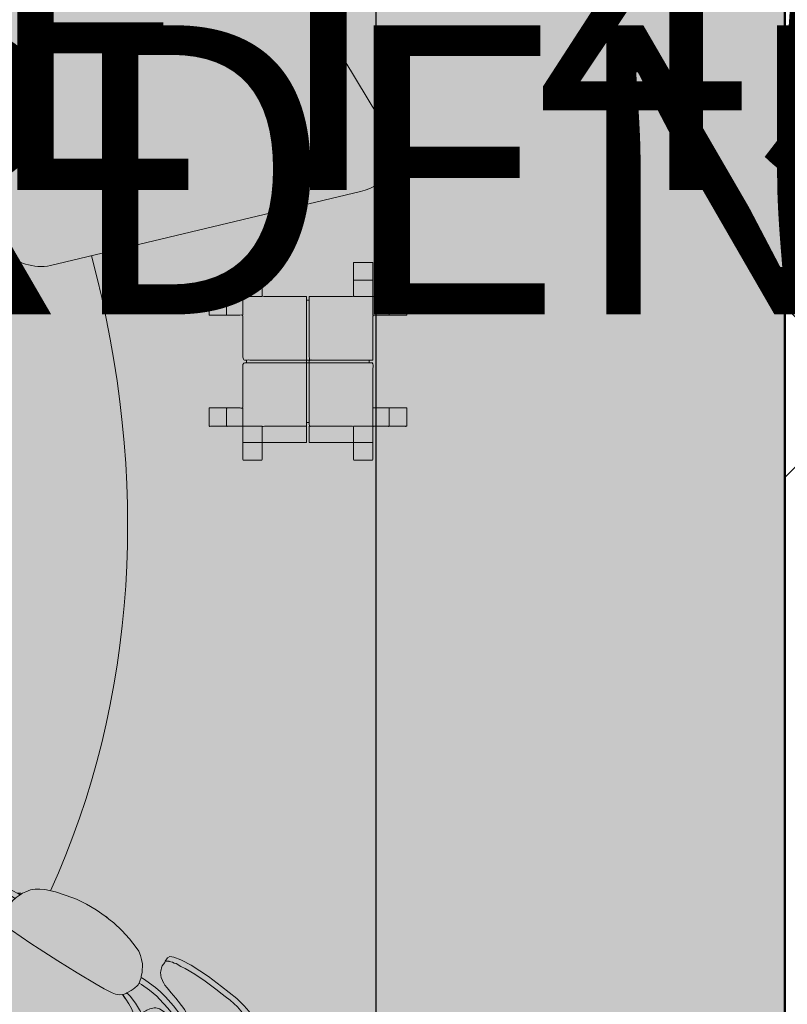
# Model space of a CAD drawing. Units: inches. Extents: x -466983 to 1020, y 324 to 318697.
# Tile 17 of 97: x 797.94 to 813.86, y 452.46 to 472.89. Entities that reach past the tile are written whole.
import ezdxf

# ---------------------------------------------------------------- set-up
doc = ezdxf.new("R2010")
doc.units = ezdxf.units.IN
doc.header["$MEASUREMENT"] = 0
for name, color, linetype, lineweight in [('A-ANNO-DIMS', 2, 'Continuous', 18), ('A-FLOR-PATT', 252, 'Continuous', 13), ('A-FURN', 8, 'Continuous', 18), ('A-WALL', 7, 'Continuous', 50)]:
    doc.layers.add(name, color=color, linetype=linetype, lineweight=lineweight)
doc.layers.add('K-Hatch', color=7, linetype='Continuous')
doc.styles.get("Standard").update_dxf_attribs({"font": 'arial.ttf'})
doc.dimstyles.get("Standard").update_dxf_attribs({"dimtxt": 6, "dimasz": 4, "dimexe": 3, "dimexo": 3, "dimgap": 0.09, "dimtad": 0, "dimtih": 1, "dimtoh": 1, "dimdec": 1, "dimzin": 0, "dimdsep": 46, "dimlunit": 3, "dimtxsty": 'Standard', "dimcen": 0.09, "dimadec": 0, "dimazin": 0, "dimtfac": 1, "dimtdec": 1, "dimtofl": 0, "dimtmove": 0, "dimatfit": 3, "dimfxl": 1, "dimtolj": 1, "dimtzin": 0, "dimarcsym": 0})

# ---------------------------------------------------------------- blocks, each defined once
blk = doc.blocks.new('CBV_09')
for points, knots in [([(-122.8, 153.5), (-122.8, 170.2), (-122.8, 186.8), (-104.5, 186.8), (-86.3, 186.8)], [99, 99, 99, 100, 100, 101, 101, 101]), ([(-122.8, 153.5), (-122.8, 170.2), (-122.8, 186.8), (-104.5, 186.8), (-86.3, 186.8)], [99, 99, 99, 100, 100, 101, 101, 101]), ([(86.3, 153.5), (86.3, 170.2), (86.3, 186.8), (104.5, 186.8), (122.8, 186.8)], [45, 45, 45, 46, 46, 47, 47, 47]), ([(86.3, 153.5), (86.3, 170.2), (86.3, 186.8), (104.5, 186.8), (122.8, 186.8)], [45, 45, 45, 46, 46, 47, 47, 47]), ([(-29.2, 122.7), (-20.7, 122.7), (-12.2, 122.7), (-7.4, 122.7), (-2.6, 122.7), (-2.6, 105.2), (-2.6, 87.7), (-2.6, 45.2), (-2.6, 2.6), (-7.4, 2.6), (-12.2, 2.6), (-20.7, 2.6), (-29.2, 2.6), (-57.8, 2.6), (-86.3, 2.6), (-104.5, 2.6), (-122.8, 2.6), (-122.8, 45.2), (-122.8, 87.7), (-138.1, 87.7), (-153.5, 87.7), (-153.5, 105.2), (-153.5, 122.7), (-138.1, 122.7), (-122.8, 122.7), (-122.8, 138.1), (-122.8, 153.5), (-104.5, 153.5), (-86.3, 153.5), (-86.3, 138.1), (-86.3, 122.7), (-57.8, 122.7), (-29.2, 122.7)], [73, 73, 73, 74, 74, 75, 75, 76, 76, 77, 77, 78, 78, 79, 79, 80, 80, 81, 81, 82, 82, 83, 83, 84, 84, 85, 85, 86, 86, 87, 87, 88, 88, 89, 89, 89]), ([(-29.2, 122.7), (-20.7, 122.7), (-12.2, 122.7), (-7.4, 122.7), (-2.6, 122.7), (-2.6, 105.2), (-2.6, 87.7), (-2.6, 45.2), (-2.6, 2.6), (-7.4, 2.6), (-12.2, 2.6), (-20.7, 2.6), (-29.2, 2.6), (-57.8, 2.6), (-86.3, 2.6), (-104.5, 2.6), (-122.8, 2.6), (-122.8, 45.2), (-122.8, 87.7), (-138.1, 87.7), (-153.5, 87.7), (-153.5, 105.2), (-153.5, 122.7), (-138.1, 122.7), (-122.8, 122.7), (-122.8, 138.1), (-122.8, 153.5), (-104.5, 153.5), (-86.3, 153.5), (-86.3, 138.1), (-86.3, 122.7), (-57.8, 122.7), (-29.2, 122.7)], [73, 73, 73, 74, 74, 75, 75, 76, 76, 77, 77, 78, 78, 79, 79, 80, 80, 81, 81, 82, 82, 83, 83, 84, 84, 85, 85, 86, 86, 87, 87, 88, 88, 89, 89, 89]), ([(29.1, 2.6), (20.6, 2.6), (12.1, 2.6), (7.3, 2.6), (2.6, 2.6), (2.6, 45.2), (2.6, 87.7), (2.6, 105.2), (2.6, 122.7), (7.3, 122.7), (12.1, 122.7), (20.6, 122.7), (29.1, 122.7), (57.7, 122.7), (86.3, 122.7), (86.3, 138.1), (86.3, 153.5), (104.5, 153.5), (122.8, 153.5), (122.8, 138.1), (122.8, 122.7)], [26, 26, 26, 27, 27, 28, 28, 29, 29, 30, 30, 31, 31, 32, 32, 33, 33, 34, 34, 35, 35, 36, 36, 36]), ([(-153.5, 87.7), (-170.2, 87.7), (-186.8, 87.7), (-186.8, 105.2), (-186.8, 122.7)], [110, 110, 110, 111, 111, 112, 112, 112]), ([(-153.5, 87.7), (-170.2, 87.7), (-186.8, 87.7), (-186.8, 105.2), (-186.8, 122.7)], [110, 110, 110, 111, 111, 112, 112, 112]), ([(-122.8, 87.7), (-122.8, 105.2), (-122.8, 122.7), (-104.5, 122.7), (-86.3, 122.7)], [0, 0, 0, 1, 1, 2, 2, 2]), ([(122.8, 122.7), (138.1, 122.7), (153.5, 122.7), (153.5, 105.2), (153.5, 87.7), (138.1, 87.7), (122.8, 87.7), (122.8, 45.2), (122.8, 2.6), (104.5, 2.6), (86.3, 2.6), (57.7, 2.6), (29.1, 2.6)], [324, 324, 324, 325, 325, 326, 326, 327, 327, 328, 328, 329, 329, 330, 330, 330]), ([(122.8, 122.7), (138.1, 122.7), (153.5, 122.7), (153.5, 105.2), (153.5, 87.7), (138.1, 87.7), (122.8, 87.7), (122.8, 45.2), (122.8, 2.6), (104.5, 2.6), (86.3, 2.6), (57.7, 2.6), (29.1, 2.6)], [324, 324, 324, 325, 325, 326, 326, 327, 327, 328, 328, 329, 329, 330, 330, 330]), ([(122.8, 87.7), (122.8, 105.2), (122.8, 122.7), (104.5, 122.7), (86.3, 122.7)], [1, 1, 1, 2, 2, 3, 3, 3]), ([(153.5, 122.7), (170.2, 122.7), (186.8, 122.7), (186.8, 105.2), (186.8, 87.7), (170.2, 87.7), (153.5, 87.7)], [314, 314, 314, 315, 315, 316, 316, 317, 317, 317]), ([(153.5, 122.7), (170.2, 122.7), (186.8, 122.7), (186.8, 105.2), (186.8, 87.7), (170.2, 87.7), (153.5, 87.7)], [314, 314, 314, 315, 315, 316, 316, 317, 317, 317]), ([(-2.6, 2.6), (-2.6, 0), (-2.6, -2.6), (0, -2.6), (2.6, -2.6)], [0.000014, 0.000014, 0.000014, 1, 1, 2, 2, 2]), ([(2.6, -2.6), (2.6, 0), (2.6, 2.6), (0, 2.6), (-2.6, 2.6)], [2, 2, 2, 3, 3, 3.999968, 3.999968, 3.999968]), ([(-122.8, -122.7), (-138.1, -122.7), (-153.5, -122.7), (-153.5, -105.2), (-153.5, -87.7), (-138.1, -87.7), (-122.8, -87.7), (-122.8, -45.2), (-122.8, -2.6), (-104.5, -2.6), (-86.3, -2.6), (-57.8, -2.6), (-29.2, -2.6), (-20.7, -2.6), (-12.2, -2.6), (-7.4, -2.6), (-2.6, -2.6)], [0, 0, 0, 1, 1, 2, 2, 3, 3, 4, 4, 5, 5, 6, 6, 7, 7, 8, 8, 8]), ([(-122.8, -122.7), (-138.1, -122.7), (-153.5, -122.7), (-153.5, -105.2), (-153.5, -87.7), (-138.1, -87.7), (-122.8, -87.7), (-122.8, -45.2), (-122.8, -2.6), (-104.5, -2.6), (-86.3, -2.6), (-57.8, -2.6), (-29.2, -2.6), (-20.7, -2.6), (-12.2, -2.6), (-7.4, -2.6), (-2.6, -2.6)], [0, 0, 0, 1, 1, 2, 2, 3, 3, 4, 4, 5, 5, 6, 6, 7, 7, 8, 8, 8]), ([(-2.6, -2.6), (-2.6, -45.2), (-2.6, -87.7), (-2.6, -105.2), (-2.6, -122.7), (-7.4, -122.7), (-12.2, -122.7), (-20.7, -122.7), (-29.2, -122.7), (-57.8, -122.7), (-86.3, -122.7), (-86.3, -138.1), (-86.3, -153.5), (-104.5, -153.5), (-122.8, -153.5), (-122.8, -138.1), (-122.8, -122.7)], [344, 344, 344, 345, 345, 346, 346, 347, 347, 348, 348, 349, 349, 350, 350, 351, 351, 352, 352, 352]), ([(153.5, -87.7), (153.5, -105.2), (153.5, -122.7), (138.1, -122.7), (122.8, -122.7), (122.8, -138.1), (122.8, -153.5), (104.5, -153.5), (86.3, -153.5), (86.3, -138.1), (86.3, -122.7), (57.7, -122.7), (29.1, -122.7), (20.6, -122.7), (12.1, -122.7), (7.3, -122.7), (2.6, -122.7), (2.6, -105.2), (2.6, -87.7), (2.6, -45.2), (2.6, -2.6), (7.3, -2.6), (12.1, -2.6), (20.6, -2.6), (29.1, -2.6), (57.7, -2.6), (86.3, -2.6), (104.5, -2.6), (122.8, -2.6), (122.8, -45.2), (122.8, -87.7)], [279.000001, 279.000001, 279.000001, 280, 280, 281, 281, 282, 282, 283, 283, 284, 284, 285, 285, 286, 286, 287, 287, 288, 288, 289, 289, 290, 290, 291, 291, 292, 292, 293, 293, 294, 294, 294]), ([(-153.5, -122.7), (-170.2, -122.7), (-186.8, -122.7), (-186.8, -105.2), (-186.8, -87.7)], [150, 150, 150, 151, 151, 152, 152, 152]), ([(-153.5, -122.7), (-170.2, -122.7), (-186.8, -122.7), (-186.8, -105.2), (-186.8, -87.7)], [150, 150, 150, 151, 151, 152, 152, 152]), ([(-122.8, -87.7), (-122.8, -105.2), (-122.8, -122.7), (-104.5, -122.7), (-86.3, -122.7)], [1, 1, 1, 2, 2, 3, 3, 3]), ([(122.8, -87.7), (122.8, -105.2), (122.8, -122.7), (104.5, -122.7), (86.3, -122.7)], [1, 1, 1, 2, 2, 3, 3, 3]), ([(153.5, -87.7), (170.2, -87.7), (186.8, -87.7), (186.8, -105.2), (186.8, -122.7), (170.2, -122.7), (153.5, -122.7)], [238, 238, 238, 239, 239, 240, 240, 241, 241, 241]), ([(153.5, -87.7), (170.2, -87.7), (186.8, -87.7), (186.8, -105.2), (186.8, -122.7), (170.2, -122.7), (153.5, -122.7)], [238, 238, 238, 239, 239, 240, 240, 241, 241, 241]), ([(-86.3, -153.5), (-86.3, -170.2), (-86.3, -186.8), (-104.5, -186.8), (-122.8, -186.8), (-122.8, -170.2), (-122.8, -153.5)], [161, 161, 161, 162, 162, 163, 163, 164, 164, 164]), ([(-86.3, -153.5), (-86.3, -170.2), (-86.3, -186.8), (-104.5, -186.8), (-122.8, -186.8), (-122.8, -170.2), (-122.8, -153.5)], [161, 161, 161, 162, 162, 163, 163, 164, 164, 164]), ([(-2.6, -153.5), (-7.4, -153.5), (-12.2, -153.5), (-20.7, -153.5), (-29.2, -153.5), (-57.8, -153.5), (-86.3, -153.5)], [258, 258, 258, 259, 259, 260, 260, 261, 261, 261]), ([(-2.6, -153.5), (-7.4, -153.5), (-12.2, -153.5), (-20.7, -153.5), (-29.2, -153.5), (-57.8, -153.5), (-86.3, -153.5)], [258, 258, 258, 259, 259, 260, 260, 261, 261, 261]), ([(86.3, -153.5), (57.7, -153.5), (29.1, -153.5), (20.6, -153.5), (12.1, -153.5), (7.3, -153.5), (2.6, -153.5)], [254, 254, 254, 255, 255, 256, 256, 257, 257, 257]), ([(86.3, -153.5), (57.7, -153.5), (29.1, -153.5), (20.6, -153.5), (12.1, -153.5), (7.3, -153.5), (2.6, -153.5)], [254, 254, 254, 255, 255, 256, 256, 257, 257, 257]), ([(122.8, -153.5), (122.8, -170.2), (122.8, -186.8), (104.5, -186.8), (86.3, -186.8), (86.3, -170.2), (86.3, -153.5)], [227, 227, 227, 228, 228, 229, 229, 230, 230, 230]), ([(122.8, -153.5), (122.8, -170.2), (122.8, -186.8), (104.5, -186.8), (86.3, -186.8), (86.3, -170.2), (86.3, -153.5)], [227, 227, 227, 228, 228, 229, 229, 230, 230, 230])]:
    blk.add_open_spline(points, degree=2, knots=knots)
for points in [[(-86.3, 186.8), (-86.3, 170.2), (-86.3, 153.5)], [(-86.3, 186.8), (-86.3, 170.2), (-86.3, 153.5)], [(122.8, 186.8), (122.8, 170.2), (122.8, 153.5)], [(122.8, 186.8), (122.8, 170.2), (122.8, 153.5)], [(-186.8, 122.7), (-170.2, 122.7), (-153.5, 122.7)], [(-186.8, 122.7), (-170.2, 122.7), (-153.5, 122.7)], [(-2.6, 115.7), (0, 115.7), (2.6, 115.7)], [(-2.6, 115.7), (0, 115.7), (2.6, 115.7)], [(2.6, 122.7), (2.6, 122.7), (2.6, 122.7)], [(2.6, 122.7), (2.6, 122.7), (2.6, 122.7)], [(-115.7, -2.6), (-115.7, 0), (-115.7, 2.6)], [(-115.7, -2.6), (-115.7, 0), (-115.7, 2.6)], [(-2.6, 2.6), (-2.6, 2.6), (-2.6, 2.6)], [(-2.6, 2.6), (-2.6, 2.6), (-2.6, 2.6)], [(115.7, 2.6), (115.7, 0), (115.7, -2.6)], [(115.7, 2.6), (115.7, 0), (115.7, -2.6)], [(115.7, 2.6), (119.2, 2.6), (122.8, 2.6)], [(115.7, 2.6), (119.2, 2.6), (122.8, 2.6)], [(-86.3, -2.6), (-86.3, -2.6), (-86.3, -2.6)], [(-86.3, -2.6), (-86.3, -2.6), (-86.3, -2.6)], [(-29.2, -2.6), (-29.2, -2.6), (-29.2, -2.6)], [(-29.2, -2.6), (-29.2, -2.6), (-29.2, -2.6)], [(-12.2, -2.6), (-12.2, -2.6), (-12.2, -2.6)], [(-12.2, -2.6), (-12.2, -2.6), (-12.2, -2.6)], [(2.6, -2.6), (2.6, -2.6), (2.6, -2.6)], [(12.1, -2.6), (12.1, -2.6), (12.1, -2.6)], [(12.1, -2.6), (12.1, -2.6), (12.1, -2.6)], [(29.1, -2.6), (29.1, -2.6), (29.1, -2.6)], [(86.3, -2.6), (86.3, -2.6), (86.3, -2.6)], [(86.3, -2.6), (86.3, -2.6), (86.3, -2.6)], [(115.7, -2.6), (115.7, -2.6), (115.7, -2.6)], [(115.7, -2.6), (115.7, -2.6), (115.7, -2.6)], [(115.7, -2.6), (119.2, -2.6), (122.8, -2.6)], [(115.7, -2.6), (119.2, -2.6), (122.8, -2.6)], [(-186.8, -87.7), (-170.2, -87.7), (-153.5, -87.7)], [(-186.8, -87.7), (-170.2, -87.7), (-153.5, -87.7)], [(122.8, -87.7), (138.1, -87.7), (153.5, -87.7)], [(122.8, -87.7), (138.1, -87.7), (153.5, -87.7)], [(2.6, -115.7), (0, -115.7), (-2.6, -115.7)], [(-2.6, -153.5), (-2.6, -138.1), (-2.6, -122.7)], [(2.6, -153.5), (2.6, -138.1), (2.6, -122.7)]]:
    blk.add_open_spline(points, degree=2)
blk = doc.blocks.new('CBV_05')
at = {"layer": 'K-Hatch'}
h = blk.add_hatch(color=256, dxfattribs=at)
h.dxf.hatch_style = 1
h.paths.add_polyline_path([(614, 437), (1251.4, 62.5), (1198.3, -263.2), (564.8, -9.8), (344.4, -5.5), (343.7, -629.7, 0.159768), (369.9, -672.6), (1020.5, -1025.6, 0.317347), (1135.5, -1017.7), (1739.5, -492.7, 0.378101), (1761.2, -362.2), (1507.4, -70.4, -0.119239), (1492.6, -25.8), (1499.5, 665.1, 0.256804), (1446.2, 745.4), (822.7, 1028.7, 0.297137), (714, 1018.3), (625, 963.6), (549.5, 1037.1), (186.8, 587.5), (-1106.2, 397.7), (-1098.6, 311.5), (-1098.4, 310.2)])
h.paths.add_polyline_path([(344.4, -5.5), (-1216.9, 24.6), (-1212.3, 260), (-1718.1, 162.7, 0.51466), (-1765.1, 50), (-1478.1, -479.5, 0.244482), (-1398.8, -526.6), (323.6, -658.2, 0.453292), (343.1, -629.8, 0.006511), (343.7, -631.8)])
blk.add_lwpolyline([(1761.2, -362.2, -0.378101), (1739.5, -492.7), (1135.5, -1017.7, -0.317347), (1020.5, -1025.6), (369.9, -672.6, -0.159481), (343.2, -630.1, -0.449095), (323.6, -658.2), (-1398.8, -526.6, -0.244482), (-1478.1, -479.5), (-1765.1, 50, -0.51466), (-1718.1, 162.7), (-1212.3, 260), (-1211.5, 301.9), (-1098.4, 310.2), (-1106.2, 397.7), (186.8, 587.5), (549.5, 1037.1), (625, 963.6), (714, 1018.3, -0.297137), (822.7, 1028.7), (1446.2, 745.4, -0.256804), (1499.5, 665.1), (1492.6, -25.8, 0.119239), (1507.4, -70.4)], format="xyb", close=True)
blk.add_lwpolyline([(-1212.3, 260), (-1718.1, 162.7, 0.51466), (-1765.1, 50), (-1478.1, -479.5, 0.244482), (-1398.8, -526.6), (323.6, -658.2)], format="xyb")
blk = doc.blocks.new('CBV_11')
at = {"layer": 'K-Hatch'}
h = blk.add_hatch(color=256, dxfattribs=at)
h.dxf.hatch_style = 1
h.paths.add_polyline_path([(-178.4, 698.3), (-200.4, 717.9), (-207.1, 720), (-213, 721.7), (-231.8, 722.5), (-254.2, 721.5), (-275, 717.7), (-289.3, 712.5), (-316, 699.4), (-324.9, 694.8), (-295.8, 706.5), (-286.8, 709.3), (-277.1, 712.2), (-265.3, 715), (-258.1, 715.9), (-241.3, 718.1), (-228.8, 718), (-215.5, 715.7), (-208.8, 713.2), (-205.5, 711.6), (-203.9, 710.6), (-202.4, 709.7), (-195.4, 705.2), (-194.8, 704.5), (-190.4, 699.8), (-87.3, 570), (16.1, 440.3), (19.6, 435), (22.9, 426.4), (24.1, 422.9), (25.8, 412.3), (25.1, 398.9), (24.2, 394.5), (25.6, 399.8), (28.8, 418.8), (27.5, 432), (13.6, 457)])
h.paths.add_polyline_path([(-536, 213.1), (-639.3, 342.7), (-642.9, 348.1), (-646.2, 356.7), (-647.4, 360.2), (-649.1, 370.8), (-648.4, 384.2), (-645.7, 396.4), (-637.3, 419.1), (-631.8, 430), (-626.9, 438.8), (-622.1, 446.9), (-606.5, 469.3), (-631, 439.9), (-638.6, 427.4), (-646.5, 408.6), (-652.3, 388), (-655.6, 368.8), (-654.4, 355.7), (-649, 343.1), (-640.5, 330.7), (-448.6, 89.4), (-437.6, 77.7), (-424.8, 69.2), (-413.8, 65.9), (-392.4, 64.7), (-388.1, 65), (-394.5, 65), (-407.8, 67.4), (-417, 71.1), (-420.9, 73.4), (-427.9, 77.9), (-428.5, 78.6), (-432.9, 83.2)])
for p, q in [((259, 150.4), (259, 150.4)), ((345.2, 98.6), (344, 99.3)), ((349.3, 96), (349.2, 96.1)), ((478.6, -6.2), (478.7, -6.3)), ((644.9, -391.7), (644.8, -391.9)), ((-99, -470.6), (-98.6, -470.7)), ((4, -570.8), (3.9, -570.4)), ((96.9, -581.8), (98.6, -582.5)), ((157.6, -594.8), (157.4, -595)), ((239.9, -716.7), (240.2, -716.7))]:
    blk.add_line(p, q)
for points in [[(9, 353), (10.3, 354.9), (16.2, 365.1), (21.5, 376.3), (26.2, 388.3), (30.1, 400.3), (33.2, 412.3), (35.5, 424.1), (35.7, 431), (33.5, 442.1), (26.2, 456.4), (21.3, 463.1), (-173.2, 707.5), (-185, 718.7), (-200.1, 726), (-205.3, 726.9), (-216.4, 727.2), (-226.1, 726.9), (-241.2, 725.8), (-253.7, 723.9), (-264.9, 721.5), (-277.2, 717.9), (-288.3, 713.3), (-311.8, 701.8), (-324.9, 694.8), (-316, 699.4), (-289.3, 712.5), (-275, 717.7), (-254.2, 721.5), (-231.8, 722.5), (-213, 721.7), (-207.1, 720), (-200.4, 717.9), (-178.4, 698.3), (13.6, 457), (27.5, 432), (28.8, 418.8), (25.6, 399.8), (24.2, 394.5)], [(-16.4, 313.8), (-16.1, 314.2), (2.3, 340.9), (8.8, 352.7), (9, 353), (14.8, 365.2), (18.6, 375.8), (20.5, 381.1), (22.4, 386.6), (24.2, 394.5), (25.1, 398.9), (25.8, 412.3), (24.1, 422.9), (22.9, 426.4), (19.6, 435), (16.1, 440.3), (-87.3, 570), (-190.4, 699.8), (-194.8, 704.5), (-195.4, 705.2), (-202.4, 709.7), (-203.9, 710.6), (-208.8, 713.2), (-215.5, 715.7), (-228.8, 718), (-241.3, 718.1), (-258.1, 715.9), (-265.3, 715), (-277.1, 712.2), (-286.8, 709.3), (-295.8, 706.5), (-324.9, 694.8), (-347.4, 685.7), (-397.3, 660.4), (-444.8, 630.8), (-480.8, 604.2), (-497.4, 590.5), (-534.5, 556.2), (-554.4, 535.5), (-590.2, 492.6), (-603.5, 473.5), (-606.5, 469.3), (-622.1, 446.9), (-626.9, 438.8), (-631.8, 430), (-637.3, 419.1), (-645.7, 396.4), (-648.4, 384.2), (-649.1, 370.8), (-647.4, 360.2), (-646.2, 356.7), (-642.9, 348.1), (-639.3, 342.7), (-536, 213.1), (-432.9, 83.2), (-428.5, 78.6), (-427.9, 77.9), (-420.9, 73.4), (-417, 71.1), (-407.8, 67.4), (-394.5, 65), (-388.1, 65), (-382, 64.9), (-376.6, 65.6), (-368.3, 66.6), (-367.7, 66.7), (-359.3, 67.5), (-346.5, 70.4), (-345.9, 70.6), (-336.1, 73.3), (-327.3, 76.2), (-282.4, 94.4), (-275.6, 97.1), (-225.7, 122.4), (-178.3, 151.9), (-142.2, 178.6), (-125.6, 192.2), (-88.5, 226.6), (-68.7, 247.3), (-32.9, 290.2), (-16.4, 313.8), (-16.2, 314.2)], [(-203.9, 710.6), (-205.5, 711.6), (-208.8, 713.2)], [(-346.5, 70.4), (-349.3, 69.2), (-356.8, 67), (-372.9, 63.3), (-385.5, 61.5), (-398.1, 60.5), (-410.3, 60.2), (-421.5, 60.6), (-428.5, 61.9), (-441.8, 68.9), (-453.7, 80.2), (-456.3, 83.2), (-648.2, 324.6), (-653.1, 331.3), (-657.2, 338.3), (-662.3, 353.4), (-662.3, 363.4), (-659.9, 375.1), (-656.8, 387), (-652.8, 399), (-648.1, 410.9), (-642.7, 422.1), (-636.8, 432.3), (-630.4, 441.2), (-607, 469.6), (-603.5, 473.5)], [(-606.5, 469.3), (-631, 439.9), (-638.6, 427.4), (-646.5, 408.6), (-652.3, 388), (-655.6, 368.8), (-654.4, 355.7), (-649, 343.1), (-640.5, 330.7), (-448.6, 89.4), (-437.6, 77.7), (-424.8, 69.2), (-413.8, 65.9), (-392.4, 64.7), (-388.1, 65)], [(-50.1, 67.5), (-23.5, 87.9), (-9.9, 97.6), (3.8, 107.1), (17.8, 116.4), (31.9, 125.3), (60.6, 142.4), (89.9, 158.3), (119.5, 173.3), (135, 179.9), (142.8, 182.8), (151, 184.8), (159.6, 185.9), (175.9, 186.9), (181, 186.7)], [(46.8, 133.3), (53.6, 137.3), (58.1, 140), (60.8, 141.6), (71.5, 147.3), (71.5, 147.3), (75.4, 149.5), (86.9, 155.7), (90, 157.4), (100.5, 162.5), (100.5, 162.6), (112.3, 168.5), (118.5, 171.5), (121.5, 172.9), (121.5, 172.9), (121.6, 172.9), (124.8, 174.4), (126.7, 175.2), (131.7, 177.5), (133.5, 178.2), (133.6, 178.2), (139.5, 180.3), (143.1, 181.6), (144.9, 182), (148.5, 182.9), (151.1, 183.5), (151.4, 183.6), (155.5, 184.6), (157.4, 184.8), (163.9, 185.7), (168.2, 186.2), (170.2, 186.3), (175.4, 186.4), (175.6, 186.4), (175.8, 186.4), (179.6, 186.5), (181.7, 186.3), (187.4, 185.9), (192.1, 185.5), (192.4, 185.5), (192.9, 185.4), (196.6, 184.9), (199.1, 184.5), (203, 183.5), (203.6, 183.4), (204.9, 183.1), (206.1, 182.8), (206.2, 182.8), (206.9, 182.5), (210.6, 181.4), (212.8, 180.8), (213.1, 180.7), (213.6, 180.5), (215.8, 179.8), (217.2, 179.4), (219, 178.7), (225, 176.1), (225.2, 176), (225.4, 175.9), (228.9, 174.4), (230.6, 173.5), (239.3, 168.6), (259, 150.4), (261.9, 146.4), (265.2, 141.7), (271.3, 132.8), (271.8, 133.4)], [(268, 169.8), (264.7, 172.2), (256.3, 176.5), (245.7, 180.3), (233.5, 183.5), (219.5, 185.8), (204.9, 187.1), (190.5, 187.3), (181, 186.7), (184.6, 186.6), (192.1, 185.5)], [(215.8, 179.8), (224.2, 178.5), (244.5, 172), (258.1, 164.6), (259.6, 163.4)], [(325.2, 88.8), (320.7, 95.5), (312.8, 106.8), (299.7, 124.6), (287.2, 140.3), (277.4, 151.6), (268.4, 160.4), (262.4, 164.5), (259.6, 163.6), (268, 169.8), (268.8, 170.4), (273.2, 169.7), (281.2, 162.9), (287.4, 156.5), (292.6, 150.4), (299.8, 141.9), (315.6, 121.4), (329.6, 101.6), (335.5, 92.9)], [(259.6, 163.6), (259.6, 163.4), (260.3, 157.9), (264.5, 147.6), (271, 134.8), (273.6, 130.4), (280, 119.4), (306, 80.1)], [(346.5, 95.7), (344, 99.3), (342.7, 101.1), (342.4, 101.6), (329.1, 118.9), (319.4, 130.1), (312.4, 136.8), (292.6, 150.4)], [(58.1, 140), (55.3, 138.4), (46.8, 133.3), (43.3, 131.2), (32.8, 125), (30.4, 123.5), (28, 122), (23.4, 119.1), (14, 112.9), (5.4, 107.3), (1.3, 104.5), (-2.9, 101.6), (-9.4, 97), (-9.5, 96.9), (-21, 88.8), (-24.8, 86), (-28.5, 83.3), (-36.4, 77.2), (-38.8, 75.4), (-45.1, 70.6), (-49.7, 67), (-54.2, 63.4), (-56, 61.9), (-62.5, 56.6), (-75.5, 45.6), (-77.3, 44), (-77.4, 44)], [(457.4, -155.4), (455.9, -155.5), (454.8, -155.5), (454.6, -155.5), (454.5, -155.5), (450.3, -155.2), (448.8, -154.8), (444.9, -153.5), (441.6, -151.7), (437.3, -148.8), (429.3, -140.4), (425.9, -136.3), (421.6, -130.7), (411.3, -116.8), (398.5, -99.2), (386.7, -82.7), (374.5, -65.3), (362.5, -47.8), (339.1, -12.8), (318.2, 19.8), (307.7, 36.3), (302.4, 46.9), (301.4, 48.8), (298.5, 55.5), (297.9, 58.1), (297.8, 65.2), (298.5, 67.6), (301, 75.1), (306, 80.1), (307.5, 81.6), (308.1, 82), (307.8, 84), (308.9, 85.7), (310.4, 86.8), (312.8, 87.1), (320.3, 87.9), (323, 87.9), (324.8, 88.6), (325.2, 88.8), (330.7, 91.3), (335.5, 92.9), (337.7, 93.7), (344.7, 95.5), (346.5, 95.7), (349.3, 96), (349.8, 96), (359.2, 96.9), (368.2, 95.8), (377.2, 93.8), (385.7, 90.7), (393.6, 86.2), (410.4, 73.5), (416, 68.7), (426.3, 59.8), (441.3, 45.2), (454.8, 29), (467.2, 12.1), (478.3, -5.7), (478.6, -6.2), (478.6, -6.3), (479, -7), (481, -10.8), (488.2, -24.1), (496, -43.4), (503.1, -63.4), (508.5, -83.5), (509.8, -91.8), (509.7, -100.3), (508.6, -108.6), (506.6, -116.7), (503.3, -124.2), (500, -131.2), (494.1, -139.1), (490.8, -143.5), (486.4, -147), (485.6, -147.6), (485.6, -147.6)], [(349.8, 96), (347.9, 98), (342.9, 101.1), (342.7, 101.1)], [(-217.7, -216.8), (-218.7, -214.8), (-221.6, -206), (-223.5, -195.1), (-224.4, -170.3), (-223.2, -156.5), (-220.9, -142.4), (-219, -134.5), (-218.9, -134.4), (-218.9, -134.2), (-217.3, -125.9), (-215.2, -117.7), (-212.7, -109.9), (-212.1, -108.4), (-207.7, -98.2), (-203.6, -90.8), (-196.4, -80.6), (-191.3, -74), (-180.9, -61.1), (-170.2, -48.3), (-159.1, -35.9), (-159.1, -35.8), (-148, -23.5), (-124.9, 0.7), (-113, 12.4), (-100.8, 23.9), (-88.5, 35.1), (-75.9, 46.2), (-63.1, 57), (-50.1, 67.5)], [(-214.7, -118), (-214.6, -117.8), (-212.4, -111.4), (-210.9, -107.7), (-210.4, -106.5), (-210.1, -105.7), (-209.4, -104.2), (-209, -103.5), (-206, -97.3), (-205.1, -95.8), (-204.7, -95), (-203.9, -93.8), (-203.5, -93.2), (-202.6, -91.5), (-202, -90.5), (-200.3, -88.1), (-199.3, -86.6), (-198.2, -84.9), (-198, -84.7), (-197.9, -84.5), (-192.8, -77.9), (-190.9, -75.4), (-190.5, -74.9), (-189.8, -74), (-186.5, -69.8), (-173.8, -54.2), (-170.7, -50.6), (-169.2, -48.8), (-167, -46.3), (-160.8, -39.1), (-147.5, -24.2), (-147.4, -24.1), (-147.3, -24), (-146.9, -23.6), (-146.4, -23.1), (-134, -9.8), (-127, -2.7), (-124.7, -0.3), (-124.4, -0.1), (-124.2, 0.2), (-123.2, 1.2), (-120.2, 4.2), (-106.2, 17.9), (-102.9, 20.9), (-101.4, 22.4), (-98.9, 24.6), (-91.9, 31.1), (-77.7, 43.7), (-77.6, 43.8), (-77.4, 44)], [(479, -7), (479.3, -7.2), (478.7, -6.3), (478.6, -6.3)], [(481, -10.8), (480.9, -9.4), (480, -8.1), (479.3, -7.2), (479.9, -7.7), (480, -8.1), (480, -8.6)], [(-212.1, -108.4), (-213.8, -111.2), (-223, -134.4), (-228.6, -157.2), (-231.3, -180.4), (-231, -201.3), (-228.1, -217.6), (-225.8, -223.3), (-226.1, -223.6), (-227.6, -226.1), (-224.9, -232.9), (-218.3, -243.6), (-212.6, -251.5), (-209.6, -255.8), (-197.1, -271.4), (-182.6, -288.2), (-173.4, -298.4), (-166.3, -306.1)], [(-143.8, -278.1), (-149.7, -271.9), (-151.2, -270.2), (-153.6, -267.6), (-153.7, -267.6), (-158.2, -262.7), (-179.1, -240.4), (-181.9, -237.4), (-184, -235.2), (-185.8, -233.2), (-188.4, -230.4), (-188.8, -230), (-189.2, -229.5), (-191, -227.5), (-192.6, -225.7), (-192.9, -225.2), (-193.3, -224.8), (-194.6, -223.3), (-196.5, -221), (-197, -220.3), (-197.5, -219.7), (-198.5, -218.3), (-200, -216.4), (-200.2, -216.2), (-201.3, -214.6), (-201.4, -214.5), (-203.2, -212), (-203.8, -211.2), (-204.4, -210.2), (-205.3, -208.8), (-206.1, -207.6), (-206.2, -207.4), (-206.3, -207.3), (-206.4, -207), (-206.6, -206.8), (-207.1, -206), (-207.5, -205.3), (-207.5, -205.2), (-207.6, -205.1), (-207.6, -205), (-208.1, -204.2), (-208.2, -204), (-208.3, -203.8), (-208.4, -203.7), (-208.7, -203.2), (-209.4, -202), (-209.4, -201.9), (-209.6, -201.7), (-210.3, -200.2), (-211.3, -198.2), (-211.5, -197.7), (-212.6, -194.8), (-213.7, -191.8), (-214, -190.9), (-215.6, -185.2), (-217, -180.3), (-217, -180.3), (-217, -180.3), (-217.6, -177.7), (-218.5, -172.7), (-218.9, -170.6), (-219, -169.1), (-219.2, -168.2), (-219.2, -167.9), (-219.3, -167.8), (-219.3, -166.9), (-219.6, -165), (-219.8, -163.4), (-220.2, -156.1), (-220.2, -148.7), (-219.6, -142.8), (-219.6, -142.2), (-219.6, -142), (-219.6, -141.7), (-219.5, -141.2), (-218.5, -134), (-217.9, -130.8), (-217.7, -129.5), (-217.7, -129.3), (-217.5, -128.7), (-217.5, -128.6), (-217.4, -128.4), (-217, -126.3), (-215, -118.8), (-214.9, -118.6), (-214.9, -118.5), (-214.7, -118), (-214.9, -118.5)], [(2.4, -563.5), (-3.3, -568.8), (-5, -573.7), (-2.4, -580.9), (5.2, -592.9), (5.7, -593.8), (18.8, -610.1), (45.9, -638.4), (68.4, -659.3), (96.5, -683.5), (112.7, -694.7), (124, -701.1), (147.3, -712), (166.9, -718.5), (179.8, -721.6), (199.9, -724.8), (239.8, -727.2), (268.3, -726.6), (296.4, -724), (325.3, -719.4), (352.9, -713), (380.3, -704.7), (407.4, -694.3), (433.1, -682.4), (458.3, -668.7), (482.6, -653.1), (505.7, -636), (542.7, -602.8), (575.4, -565.6), (602.5, -526.6), (625.7, -483.1), (643.9, -436.4), (652.7, -404.6), (661, -358.1), (662.3, -341.6), (662.3, -324.4), (657.8, -289.7), (648.3, -258), (641.9, -243.3), (624.1, -210.4), (611.5, -188.5), (598.9, -168.7), (586.8, -151.4), (569.2, -131.1), (563.8, -126.7), (556, -124), (545.5, -130.4)], [(155.2, -596.2), (151.6, -595.8), (147.4, -595.1), (129.4, -592.1), (123.7, -590.8), (98.6, -582.5), (97.8, -582.2), (96.9, -581.8), (74.8, -570.5), (62.9, -563.8), (52.4, -557.5), (46.9, -554.5), (42.7, -553), (37.7, -551.6), (36.8, -551.4), (31.7, -550), (21.6, -550.8), (19.3, -551.6), (10.7, -555.3), (9.9, -555.9), (4.7, -561.9), (2.4, -563.5), (3.7, -570.3), (4, -570.8), (6.8, -576.4), (8.9, -579.3), (10.2, -583.1), (17.3, -590.8), (22.7, -598.1), (36.7, -613.8), (53.2, -630.5), (71.6, -647.7), (77.1, -652.5), (77.9, -653.2), (88.3, -662.3), (97.4, -670.5), (112.3, -681.7), (138.1, -696.5), (170, -708.5), (185.7, -712.2), (201.4, -714.5), (240.2, -716.9), (281.9, -715.3), (330.8, -707.8), (377.8, -694.8), (416.2, -679.4), (459.2, -656.3), (499.4, -628.1), (521, -609.6), (541.3, -589.7), (560.1, -568.5), (577.1, -546.4), (593, -522.5), (607, -498.1), (619.2, -472.7), (629.8, -445.9), (638.3, -419.5), (645, -392), (649.6, -365.8), (651.8, -341.4), (651.9, -325.2), (649.9, -305.2), (646.3, -287), (640.9, -268.7), (640.2, -267.3), (639, -264.2), (633.6, -250.9), (617.4, -220.5), (602.1, -193.8), (587.3, -171.3), (580.6, -161.1), (567.7, -144.8), (566, -143.1), (564.1, -141.2), (554.6, -132.1), (554, -131.9), (550.5, -130.5), (549.7, -130.2), (547.6, -129.3), (545.5, -130.4), (545.4, -130.9), (538.4, -135.5), (532.9, -143.1), (531.5, -145.1), (528.5, -154.8), (529, -166.6), (529.5, -170.7), (531.1, -176.4), (534.9, -188.3), (538.2, -199.2), (543, -215.6), (547.1, -240.2), (547.6, -254.2), (546.4, -277.3), (546.2, -281.9), (545.7, -285.4), (545.4, -287.9), (545.4, -287.9), (545.3, -288.8), (545.3, -289.2), (544.3, -296.8), (542.7, -303.6), (537, -331.4), (528.9, -353.7)], [(549.7, -130.2), (547, -129.8), (545.4, -130.9)], [(457.4, -155.4), (457.4, -155.4), (466.4, -154.5), (471.9, -153.3), (475.6, -151.4), (481.8, -150.7), (486.4, -147), (489.4, -151.4), (501.8, -172.4), (506.9, -183.2), (511.5, -194.8), (517.3, -212.7), (523.5, -234.6), (529.9, -258.9), (536.2, -278.2), (545.2, -290)], [(494.1, -139.1), (498.2, -145.2), (508.4, -161.7), (516.9, -179.1), (519.8, -186.7), (527.6, -210), (534, -233), (538.1, -249.1), (543.9, -270.8), (546.4, -277.4)], [(454.6, -155.5), (454.7, -155.7), (455.1, -157.8), (455.5, -160), (455.6, -160.6), (455.6, -160.7), (456.7, -166.6), (457.5, -171.5), (458.2, -182.7), (458.6, -192.3), (458.1, -202.7), (457.9, -204.1)], [(461.9, -154.9), (462.2, -156.4), (462.6, -158.7), (462.7, -159.1), (462.7, -159.3), (463.8, -165.3), (464.7, -170.7), (465.4, -182.4), (465.8, -192.3), (465.4, -201.6)], [(-225.8, -223.3), (-218.8, -216.5), (-217.7, -216.8), (-213.1, -218.1), (-195.7, -231.2), (-175.3, -250.4), (-147.2, -280.1)], [(-159.9, -297.1), (-165.4, -291.2), (-181.5, -273.1), (-197.1, -254.2), (-203.8, -245.5), (-213.9, -230.9), (-219, -220.9), (-218.8, -216.5)], [(-212.6, -251.5), (-211.9, -253), (-204.6, -272.1), (-201.7, -277.7), (-192.5, -291.1), (-180.6, -305.8), (-175.6, -311.7), (-173.4, -314.3), (-171.3, -316.5)], [(49.6, -472.3), (49.5, -472.3), (49.1, -466.8), (46.3, -459.7), (42.7, -453.8), (36.7, -445.8), (32.2, -440.3), (21, -427.2), (-6.6, -395.6), (-20.8, -379.7), (-35.2, -364.1), (-64.1, -333.5), (-77.2, -319.8), (-92.5, -304.3), (-108.7, -288.6), (-115.6, -282.9), (-121.5, -278.5), (-131.9, -275.3), (-141.2, -276.5), (-143.8, -278.1), (-147.2, -280.1), (-148.4, -280.8), (-149.5, -281.9), (-150.1, -282.4), (-156.3, -292.9), (-159.1, -296.2), (-158.4, -292.9), (-155.5, -285.3), (-153.9, -281.9), (-151.3, -281.2), (-149.5, -281.9)], [(59.4, -477), (56.9, -476.1), (53.2, -474.4), (49.6, -472.8), (49.7, -473.8), (48.7, -479.4), (48, -481.2), (44.9, -489.9), (42.9, -494.4), (41, -497.8), (38.6, -502.4), (37.3, -504.2), (36.9, -504.7), (34.8, -506.8), (33.8, -507.4), (29.1, -510.5), (24.1, -512.8), (22.1, -513.7), (15.1, -516.8), (-0.5, -520.1), (-9, -519.9), (-17.2, -519.3), (-25.5, -517.5), (-33.3, -514.4), (-51.7, -504.6), (-69.5, -493.5), (-86.6, -481.2), (-95.4, -473.4), (-97.6, -471.5), (-98, -471.2), (-98.6, -470.7), (-101.4, -468.2), (-101.5, -468.1), (-102.3, -467.4), (-117.4, -452.7), (-131.1, -436.8), (-143.6, -419.9), (-154.4, -402.1), (-164.5, -383.6), (-172.5, -364.3), (-175.2, -355.6), (-176.8, -346.5), (-176.8, -337.4), (-175.1, -328.4), (-173.5, -321.4), (-172.7, -319.6), (-171.3, -316.5), (-167.5, -308.1), (-166.3, -306.1), (-163.8, -301.8), (-160.2, -297.5), (-159.9, -297.1), (-159.1, -296.2)], [(545.7, -285.4), (544.3, -287.1), (544, -287.5), (543.6, -287.7), (543.5, -287.7)], [(-175.6, -311.7), (-175.4, -312.6), (-174, -317.8), (-172.7, -319.6)], [(528.6, -354.6), (528.9, -353.7), (522.8, -365.4), (515.7, -377.3), (508.1, -388.2), (503.2, -394.5), (496, -403.1), (483, -417.1), (469.3, -430.9), (454.9, -444.7), (425.1, -471.8), (395, -496.8), (363.8, -520.6), (330.7, -543.5), (314.1, -554.4), (297.5, -564.7), (281, -574.1), (263.9, -582.5), (251.4, -587.6), (244.7, -589.7), (224.5, -595.3), (204.1, -597.7), (165.9, -597.3), (155.2, -596.2), (157.4, -595), (157.2, -592.9), (152.6, -587.1)], [(-101.4, -468.2), (-100.6, -469.4), (-101.3, -468.7), (-101.5, -468.1)], [(-98, -471.2), (-98.4, -471.1), (-98.9, -470.8), (-99.9, -470.3), (-100.5, -469.5), (-100.6, -469.4)], [(-97.6, -471.5), (-98.3, -471.4), (-98.9, -470.8)], [(90.8, -500.6), (86.1, -499.5), (84, -498.9), (73.3, -495), (70.3, -493.8), (55.2, -486.1), (48, -481.2)], [(99.2, -488.5), (98.9, -488.4), (88.6, -486.6), (78.5, -484.1), (68.6, -480.9), (59.4, -477), (58.2, -476.5), (57.8, -476.3), (49.6, -472.3), (49.6, -472.3), (49.6, -472.4), (49.6, -472.4), (49.6, -472.5), (49.6, -472.8)], [(147.4, -595.1), (145, -593.4), (134.3, -587.3), (109, -574.1), (88.3, -563.1), (68.7, -551.4), (57.7, -543.9), (47.9, -536.1), (44.1, -532.6), (29.2, -518.3), (24.1, -512.8), (24.1, -512.8)], [(33.8, -507.4), (37.2, -511.1), (50.6, -524.3), (64.4, -535.5), (70.8, -539.8), (90.6, -552.1), (111.2, -563.3), (124.8, -570.5), (137.6, -577.4), (152.6, -587)]]:
    blk.add_lwpolyline(points)
blk.add_lwpolyline([(536.2, -278.2, 0.060196), (503, -207.6), (501.6, -205.9), (497.9, -203.4), (490.4, -200.5), (481.7, -199.9), (471.1, -200.5), (466.7, -201.3), (465.7, -201.5), (464.5, -201.7), (461.1, -203), (457.9, -204.1), (457.5, -204.3), (457.5, -204.3), (454.5, -205.4), (446.6, -210), (444.1, -211.8), (435.9, -217.8), (427.5, -225.4), (419.3, -234.2), (396.7, -256.7), (369.9, -282.9), (360.7, -294.8), (359, -297.1), (344.2, -313.2), (323.9, -333.2), (301.6, -353), (288.9, -363.5), (265.5, -381.1), (241.1, -397.6), (216.3, -412.6), (192.3, -424.2), (160.7, -444.5), (123.2, -467.5), (113.9, -474), (106.2, -480.6), (103.9, -482.6), (100.1, -487.3), (99.2, -488.5), (96.5, -492), (94.1, -495.1), (91.8, -498.2), (91.4, -499.3), (90.8, -500.6), (90.3, -501.9), (88.1, -510.2), (87, -512.3), (85.3, -518.2), (85.1, -527), (85.8, -529.8), (88.9, -536.1, 0.065332), (140.4, -579.1)], format="xyb")
blk = doc.blocks.new('Garden Sofa')
at = {"extrusion": (0, 0, -1)}
blk.add_ellipse((2450.434, 828.917), major_axis=(18.681, -14.923), ratio=0.833526, start_param=5.436185, end_param=6.075512, dxfattribs=at)
at = {"xscale": -0.0109740885734132, "yscale": 0.0109740885734132, "zscale": 0.0109740885734132}
for name, p, rotation in [('CBV_05', (2464.355, 846.083), 311.9356943688126), ('CBV_11', (2467.574, 814.959), 100.5267845499335)]:
    blk.add_blockref(name, p, dxfattribs=dict(at, rotation=rotation))
at = {"xscale": 0.0109740885734132, "yscale": 0.0109740885734132, "zscale": 0.0109740885734132}
blk.add_blockref('CBV_09', (2476.615, 828.512), dxfattribs=at)
blk = doc.blocks.new('*D93')
at = {"layer": 'A-ANNO-DIMS', "color": 0, "lineweight": -2, "transparency": 16777216}
for p, q in [((808.966, 500.777), (818.266, 500.777)), ((815.266, 496.777), (815.266, 472.969)), ((815.266, 442.777), (815.266, 466.584)), ((808.966, 438.777), (818.266, 438.777))]:
    blk.add_line(p, q, dxfattribs=at)
at = {"layer": 'A-ANNO-DIMS', "color": 0, "transparency": 16777216}
for points in [[(814.599, 496.777), (815.933, 496.777), (815.266, 500.777)], [(814.599, 442.777), (815.933, 442.777), (815.266, 438.777)]]:
    blk.add_solid(points, dxfattribs=at)
at = {"layer": 'Defpoints', "color": 0, "transparency": 16777216}
for p in [(805.966, 500.777), (815.266, 500.777), (805.966, 438.777)]:
    blk.add_point(p, dxfattribs=at)
at = {"layer": 'A-ANNO-DIMS', "color": 0, "transparency": 16777216, "insert": (815.266, 469.777), "char_height": 6, "attachment_point": 5}
blk.add_mtext('\\A1;GARDEN SEAT 62', dxfattribs=at)
blk = doc.blocks.new('*D97')
at = {"layer": 'A-ANNO-DIMS', "color": 0, "lineweight": -2, "transparency": 16777216}
for p, q in [((823.929, 568.441), (802.329, 568.441)), ((805.329, 564.441), (805.329, 499.545)), ((805.329, 428.441), (805.329, 493.337)), ((823.929, 424.441), (802.329, 424.441))]:
    blk.add_line(p, q, dxfattribs=at)
at = {"layer": 'A-ANNO-DIMS', "color": 0, "transparency": 16777216}
for points in [[(804.662, 564.441), (805.996, 564.441), (805.329, 568.441)], [(804.662, 428.441), (805.996, 428.441), (805.329, 424.441)]]:
    blk.add_solid(points, dxfattribs=at)
at = {"layer": 'Defpoints', "color": 0, "transparency": 16777216}
for p in [(826.929, 568.441), (805.329, 424.441), (826.929, 424.441)]:
    blk.add_point(p, dxfattribs=at)
at = {"layer": 'A-ANNO-DIMS', "color": 0, "transparency": 16777216, "insert": (805.329, 496.441), "char_height": 6, "attachment_point": 5}
blk.add_mtext('\\A1;BIKE 144', dxfattribs=at)
blk = doc.blocks.new('*D113')
at = {"layer": 'A-ANNO-DIMS', "color": 0, "lineweight": -2, "transparency": 16777216}
for p, q in [((704.71, 504.652), (709.525, 509.413)), ((710.204, 504.46), (736.319, 478.049)), ((736.45, 472.553), (741.265, 477.314)), ((739.132, 475.204), (741.944, 472.36)), ((741.944, 472.36), (745.944, 472.36))]:
    blk.add_line(p, q, dxfattribs=at)
at = {"layer": 'A-ANNO-DIMS', "color": 0, "transparency": 16777216}
for points in [[(710.678, 504.928), (709.73, 503.991), (707.392, 507.304)], [(736.794, 478.517), (735.845, 477.58), (739.132, 475.204)]]:
    blk.add_solid(points, dxfattribs=at)
at = {"layer": 'Defpoints', "color": 0, "transparency": 16777216}
for p in [(702.577, 502.543), (739.132, 475.204), (734.317, 470.443)]:
    blk.add_point(p, dxfattribs=at)
at = {"layer": 'A-ANNO-DIMS', "color": 0, "transparency": 16777216, "insert": (783.502, 472.36), "char_height": 6, "attachment_point": 5}
blk.add_mtext('\\A1;TEA TABLE SET 45', dxfattribs=at)

msp = doc.modelspace()

# ---------------------------------------------------------------- hatches: boundary and pattern name
at = {"layer": 'A-FLOR-PATT', "transparency": 33554572}
h = msp.add_hatch(dxfattribs=at)
h.set_pattern_fill('AR-HBONE', color=256, scale=3)
h.set_pattern_definition([(45, (-1212.414, -290.035), (0, 16.97056), [36, -12]), (135, (-1203.928, -281.55), (1e-15, 16.97056), [36, -12])])
h.paths.add_polyline_path([(987.806, 618.938), (813.806, 618.938), (813.806, 368.938), (987.806, 368.938)])
at = {"layer": 'A-FLOR-PATT', "transparency": 33554661}
h = msp.add_hatch(color=256, dxfattribs=at)
h.dxf.hatch_style = 1
h.set_gradient(color1=(19, 155, 72), color2=(0, 107, 0), name='CYLINDER')
h.paths.add_polyline_path([(813.806, 503.938), (730.806, 503.938), (730.806, 424.938), (612.806, 424.938), (612.806, 415.938), (442.806, 415.938), (442.806, 368.938), (813.806, 368.938)])
h.paths.add_polyline_path([(771.796, 407.07), (783.796, 407.07), (783.796, 371.07), (771.796, 371.07)], flags=16)
h.paths.add_polyline_path([(755.796, 407.07), (755.796, 371.07), (743.796, 371.07), (743.796, 407.07)], flags=16)
h.paths.add_polyline_path([(769.796, 404.07), (769.796, 374.07), (757.796, 374.07), (757.796, 404.07)], flags=16)
h.paths.add_polyline_path([(785.796, 404.07), (797.796, 404.07), (797.796, 374.07), (785.796, 374.07)], flags=16)
h.paths.add_polyline_path([(741.796, 404.07), (741.796, 374.07), (729.796, 374.07), (729.796, 404.07)], flags=16)
h.paths.add_polyline_path([(799.796, 407.07), (811.796, 407.07), (811.796, 371.07), (799.796, 371.07)], flags=16)
h.paths.add_polyline_path([(727.796, 407.07), (727.796, 371.07), (715.796, 371.07), (715.796, 407.07)], flags=16)
h.paths.add_polyline_path([(713.796, 404.07), (713.796, 374.07), (701.796, 374.07), (701.796, 404.07)], flags=16)
h.paths.add_polyline_path([(699.796, 407.07), (699.796, 371.07), (687.796, 371.07), (687.796, 407.07)], flags=16)
h.paths.add_polyline_path([(685.796, 404.07), (685.796, 374.07), (673.796, 374.07), (673.796, 404.07)], flags=16)
h.paths.add_polyline_path([(671.796, 407.07), (671.796, 371.07), (659.796, 371.07), (659.796, 407.07)], flags=16)
h.paths.add_polyline_path([(657.796, 404.07), (657.796, 374.07), (645.796, 374.07), (645.796, 404.07)], flags=16)
h.paths.add_polyline_path([(643.796, 407.07), (643.796, 371.07), (631.796, 371.07), (631.796, 407.07)], flags=16)
h.paths.add_polyline_path([(629.796, 404.07), (629.796, 374.07), (617.796, 374.07), (617.796, 404.07)], flags=16)
h.paths.add_polyline_path([(615.796, 407.07), (615.796, 371.07), (603.796, 371.07), (603.796, 407.07)], flags=16)
h.paths.add_polyline_path([(601.796, 404.07), (601.796, 374.07), (589.796, 374.07), (589.796, 404.07)], flags=16)
at = {"layer": 'A-FLOR-PATT'}
h = msp.add_hatch(dxfattribs=at)
h.set_pattern_fill('GRASS', color=256, scale=6)
h.set_pattern_definition([(90, (-1212.4137, -290.035), (-4.242641, 4.242641), [1.125, -7.360281]), (45, (-1212.4137, -290.035), (-4.24264, 4.24264), [1.125, -4.875]), (135, (-1212.4137, -290.035), (-4.24264, -4.24264), [1.125, -4.875])])
h.paths.add_polyline_path([(813.806, 503.938), (730.806, 503.938), (730.806, 424.938), (612.806, 424.938), (612.806, 415.938), (442.806, 415.938), (442.806, 368.938), (813.806, 368.938)])
h.paths.add_polyline_path([(589.796, 404.07), (601.796, 404.07), (601.796, 374.07), (589.796, 374.07)], flags=16)
h.paths.add_polyline_path([(603.796, 407.07), (615.796, 407.07), (615.796, 371.07), (603.796, 371.07)], flags=16)
h.paths.add_polyline_path([(617.796, 404.07), (629.796, 404.07), (629.796, 374.07), (617.796, 374.07)], flags=16)
h.paths.add_polyline_path([(631.796, 407.07), (643.796, 407.07), (643.796, 371.07), (631.796, 371.07)], flags=16)
h.paths.add_polyline_path([(645.796, 404.07), (657.796, 404.07), (657.796, 374.07), (645.796, 374.07)], flags=16)
h.paths.add_polyline_path([(659.796, 407.07), (671.796, 407.07), (671.796, 371.07), (659.796, 371.07)], flags=16)
h.paths.add_polyline_path([(673.796, 404.07), (685.796, 404.07), (685.796, 374.07), (673.796, 374.07)], flags=16)
h.paths.add_polyline_path([(687.796, 407.07), (699.796, 407.07), (699.796, 371.07), (687.796, 371.07)], flags=16)
h.paths.add_polyline_path([(701.796, 404.07), (713.796, 404.07), (713.796, 374.07), (701.796, 374.07)], flags=16)
h.paths.add_polyline_path([(715.796, 407.07), (727.796, 407.07), (727.796, 371.07), (715.796, 371.07)], flags=16)
h.paths.add_polyline_path([(729.796, 404.07), (741.796, 404.07), (741.796, 374.07), (729.796, 374.07)], flags=16)
h.paths.add_polyline_path([(743.796, 407.07), (755.796, 407.07), (755.796, 371.07), (743.796, 371.07)], flags=16)
h.paths.add_polyline_path([(757.796, 404.07), (769.796, 404.07), (769.796, 374.07), (757.796, 374.07)], flags=16)
h.paths.add_polyline_path([(771.796, 407.07), (783.796, 407.07), (783.796, 371.07), (771.796, 371.07)], flags=16)
h.paths.add_polyline_path([(785.796, 404.07), (797.796, 404.07), (797.796, 374.07), (785.796, 374.07)], flags=16)
h.paths.add_polyline_path([(799.796, 407.07), (811.796, 407.07), (811.796, 371.07), (799.796, 371.07)], flags=16)

# ---------------------------------------------------------------- linework, layer by layer
at = {"layer": 'A-WALL'}
msp.add_line((813.806, 618.938), (813.806, 368.938), dxfattribs=at)

# ---------------------------------------------------------------- block references
at = {"layer": 'A-FURN'}
msp.add_blockref('Garden Sofa', (-1672.7, -362.711), dxfattribs=at)

# ---------------------------------------------------------------- dimensions: what is measured, and where the dimension line sits
at = {"layer": 'A-ANNO-DIMS'}
for base, p1, p2, angle, text, picture, middle in [((805.329, 424.441), (826.929, 568.441), (826.929, 424.441), 270, 'BIKE <>', '*D97', (805.329, 496.441)), ((739.132, 475.204), (702.577, 502.543), (734.317, 470.443), 314.6775, 'TEA TABLE SET <>', '*D113', (783.502, 472.36)), ((815.266, 500.777), (805.966, 438.777), (805.966, 500.777), 90, 'GARDEN SEAT <>', '*D93', (815.266, 469.777))]:
    dim = msp.add_linear_dim(base=base, p1=p1, p2=p2, angle=angle, text=text, dimstyle='Standard', override={"dimdec": 0, "dimlfac": 1, "dimrnd": 0, "dimzin": 0, "dimdsep": 46, "dimlunit": 2}, dxfattribs=at)
    dim.commit()
    dim.dimension.update_dxf_attribs({"geometry": picture, "text_midpoint": middle})

doc.saveas('drawing.dxf')
